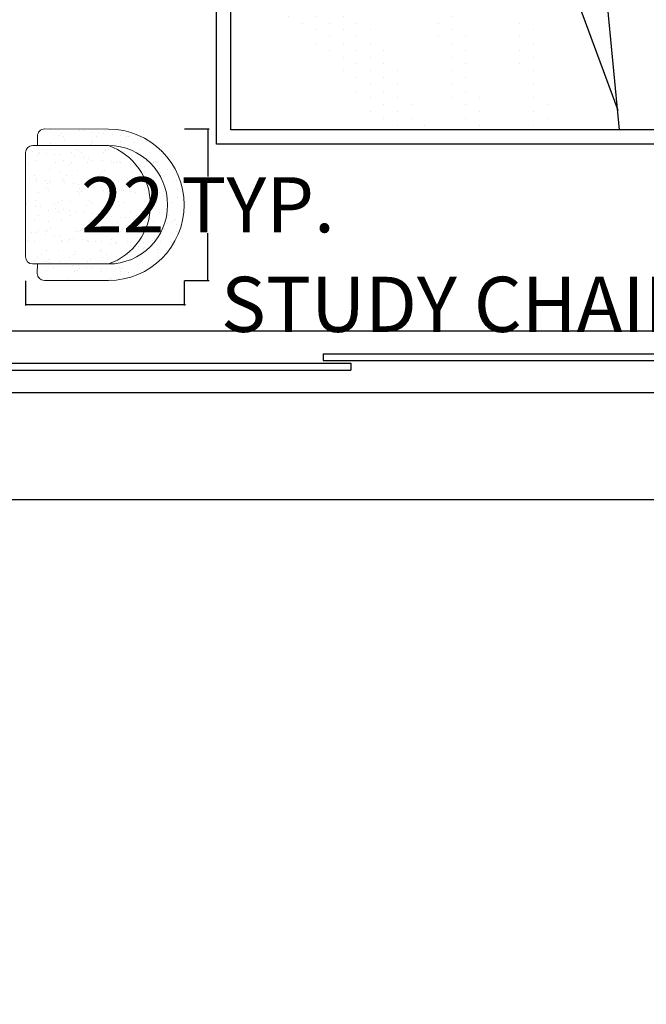
# Model space of a CAD drawing. Units: inches. Extents: x -48 to 50072, y 0 to 21068.
# Tile 60 of 75: x 793 to 883, y 660 to 803. Entities that reach past the tile are written whole.
import ezdxf

# ---------------------------------------------------------------- set-up
doc = ezdxf.new("R2010")
doc.units = ezdxf.units.IN
doc.header["$MEASUREMENT"] = 0
for name, color, linetype, lineweight in [('A-ANNO-DIMS', 2, 'Continuous', 18), ('A-DOOR', 4, 'Continuous', 18), ('FURNITURE', 44, 'Continuous', 18)]:
    doc.layers.add(name, color=color, linetype=linetype, lineweight=lineweight)
doc.layers.add('Layer3', color=176, linetype='Continuous')
doc.styles.get("Standard").update_dxf_attribs({"font": 'arial.ttf'})
doc.dimstyles.get("Standard").update_dxf_attribs({"dimtxt": 8, "dimasz": 0.18, "dimexe": 0.18, "dimexo": 0.0625, "dimgap": 0.09, "dimtad": 0, "dimtih": 1, "dimtoh": 1, "dimdec": 1, "dimzin": 0, "dimdsep": 46, "dimlunit": 4, "dimtxsty": 'Standard', "dimblk": 'ARCHTICK', "dimcen": 0.09, "dimadec": 0, "dimazin": 0, "dimtfac": 1, "dimtdec": 1, "dimtofl": 0, "dimtmove": 0, "dimatfit": 3, "dimldrblk": 'ARCHTICK', "dimfxl": 1, "dimtolj": 1, "dimtzin": 0, "dimarcsym": 0})

# ---------------------------------------------------------------- blocks, each defined once
blk = doc.blocks.new('fdsghhhhhhygr')
for p, q in [((41.77, 686.77), (41.77, 677.77)), ((144.77, 677.77), (144.77, 686.77))]:
    blk.add_line(p, q)
at = {"layer": 'Defpoints'}
for p, q in [((91.27, 683.47), (144.77, 683.47)), ((91.27, 683.47), (91.27, 682.47)), ((91.27, 682.47), (144.77, 682.47)), ((41.77, 682.07), (95.27, 682.07)), ((41.77, 681.07), (95.27, 681.07)), ((95.27, 682.07), (95.27, 681.07))]:
    blk.add_line(p, q, dxfattribs=at)
at = {"layer": 'Layer3'}
for p, q in [((41.77, 686.77), (144.77, 686.77)), ((144.77, 677.77), (41.77, 677.77))]:
    blk.add_line(p, q, dxfattribs=at)
blk = doc.blocks.new('nhrygfdu7yu')
at = {"layer": 'Defpoints'}
for p, q in [((1019.17, 828.61), (845.97, 828.61)), ((845.97, 801.61), (845.97, 828.61)), ((848.67, 804.31), (848.67, 828.61)), ((881.27, 716.83), (881.27, 828.61)), ((983.87, 828.61), (983.87, 716.83)), ((1016.47, 804.31), (1016.47, 828.61)), ((1019.17, 801.61), (1019.17, 828.61)), ((884.03, 719.53), (884.03, 827.53)), ((884.03, 827.53), (981.17, 827.53)), ((981.17, 827.53), (981.17, 719.53)), ((864.18, 805.04), (864.18, 824.84)), ((1000.24, 805.98), (1000.24, 825.78)), ((892.12, 822.13), (892.12, 801.97)), ((929.67, 822.13), (892.12, 822.13)), ((929.67, 822.13), (929.67, 801.78)), ((935.52, 822.13), (935.52, 801.78)), ((935.52, 822.13), (973.07, 822.13)), ((973.07, 822.13), (973.07, 801.97)), ((926.47, 818.07), (927.21, 812.5)), ((947.88, 818.06), (943.61, 812.45)), ((1010.72, 815.93), (989.15, 815.93)), ((874.65, 814.99), (853.09, 814.99)), ((927.21, 812.5), (925.82, 805.91)), ((934.43, 807.75), (933.36, 812.55)), ((943.61, 812.45), (939.55, 805.41)), ((914.58, 810.18), (913.28, 809.99)), ((919.69, 808.14), (914.58, 810.18)), ((923.4, 803.12), (919.69, 808.14)), ((935.49, 804.66), (934.43, 807.75)), ((881.07, 804.31), (848.67, 804.31)), ((881.07, 804.31), (881.07, 804.31)), ((916.07, 804.42), (910.77, 803.49)), ((919.78, 804.61), (916.07, 804.42)), ((923.4, 803.12), (919.78, 804.61)), ((925.82, 805.91), (923.4, 803.12)), ((938.59, 802.42), (935.49, 804.66)), ((939.55, 805.41), (938.59, 802.42)), ((938.59, 802.42), (945.53, 804.13)), ((945.53, 804.13), (951.08, 803.38)), ((984.07, 804.31), (1016.47, 804.31)), ((984.07, 804.31), (984.07, 804.31)), ((910.77, 803.49), (910.59, 803.15)), ((923.4, 803.12), (925.08, 798.67)), ((923.4, 803.12), (933.44, 802.1)), ((935.45, 803.17), (936.69, 800.13)), ((938.59, 802.42), (937.95, 797.34)), ((938.59, 802.42), (941.26, 799.01)), ((951.08, 803.38), (953.02, 802.3)), ((881.07, 801.61), (845.97, 801.61)), ((884.06, 801.97), (981.18, 801.97)), ((933.44, 802.1), (936.13, 800.15)), ((984.07, 801.61), (1019.17, 801.61)), ((925.08, 798.67), (923.96, 794.21)), ((936.13, 800.15), (936.78, 799.69)), ((936.69, 800.13), (937.65, 797.78)), ((941.26, 799.01), (944.78, 796.45)), ((937.86, 796.54), (937.22, 791.44)), ((944.78, 796.45), (949.8, 796.45)), ((981.13, 793.06), (883.98, 783.7)), ((923.96, 794.21), (921.07, 790.83)), ((906.36, 766.47), (977.44, 792.73)), ((976.41, 779.36), (976.41, 779.36)), ((978.98, 779.36), (978.98, 779.36)), ((962.27, 776.79), (962.27, 776.79)), ((964.84, 776.79), (964.84, 776.79)), ((967.41, 776.79), (967.41, 776.79)), ((969.98, 776.79), (969.98, 776.79)), ((972.55, 776.79), (972.55, 776.79)), ((975.13, 776.79), (975.13, 776.79)), ((977.7, 776.79), (977.7, 776.79)), ((980.27, 776.79), (980.27, 776.79)), ((950.69, 774.21), (950.69, 774.21)), ((953.27, 774.21), (953.27, 774.21)), ((955.84, 774.21), (955.84, 774.21)), ((958.41, 774.21), (958.41, 774.21)), ((960.98, 774.21), (960.98, 774.21)), ((963.55, 774.21), (963.55, 774.21)), ((966.13, 774.21), (966.13, 774.21)), ((968.7, 774.21), (968.7, 774.21)), ((941.69, 771.64), (941.69, 771.64)), ((944.27, 771.64), (944.27, 771.64)), ((946.84, 771.64), (946.84, 771.64)), ((949.41, 771.64), (949.41, 771.64)), ((951.98, 771.64), (951.98, 771.64)), ((954.55, 771.64), (954.55, 771.64)), ((935.26, 769.07), (935.26, 769.07)), ((937.84, 769.07), (937.84, 769.07)), ((940.41, 769.07), (940.41, 769.07)), ((942.98, 769.07), (942.98, 769.07)), ((928.83, 766.5), (928.83, 766.5)), ((931.41, 766.5), (931.41, 766.5)), ((933.98, 766.5), (933.98, 766.5)), ((936.55, 766.5), (936.55, 766.5)), ((975.13, 766.5), (975.13, 766.5)), ((977.7, 766.5), (977.7, 766.5)), ((980.27, 766.5), (980.27, 766.5)), ((924.98, 763.93), (924.98, 763.93)), ((927.55, 763.93), (927.55, 763.93)), ((930.12, 763.93), (930.12, 763.93)), ((963.55, 763.93), (963.55, 763.93)), ((966.13, 763.93), (966.13, 763.93)), ((968.7, 763.93), (968.7, 763.93)), ((971.27, 763.93), (971.27, 763.93)), ((973.84, 763.93), (973.84, 763.93)), ((976.41, 763.93), (976.41, 763.93)), ((978.98, 763.93), (978.98, 763.93)), ((921.12, 761.35), (921.12, 761.35)), ((923.69, 761.35), (923.69, 761.35)), ((954.55, 761.35), (954.55, 761.35)), ((957.12, 761.35), (957.12, 761.35)), ((959.7, 761.35), (959.7, 761.35)), ((962.27, 761.35), (962.27, 761.35)), ((964.84, 761.35), (964.84, 761.35)), ((967.41, 761.35), (967.41, 761.35)), ((969.98, 761.35), (969.98, 761.35)), ((972.55, 761.35), (972.55, 761.35)), ((975.13, 761.35), (975.13, 761.35)), ((917.26, 758.78), (917.26, 758.78)), ((919.83, 758.78), (919.83, 758.78)), ((945.55, 758.78), (945.55, 758.78)), ((948.12, 758.78), (948.12, 758.78)), ((950.69, 758.78), (950.69, 758.78)), ((953.27, 758.78), (953.27, 758.78)), ((955.84, 758.78), (955.84, 758.78)), ((958.41, 758.78), (958.41, 758.78)), ((960.98, 758.78), (960.98, 758.78)), ((963.55, 758.78), (963.55, 758.78)), ((913.4, 756.21), (913.4, 756.21)), ((915.98, 756.21), (915.98, 756.21)), ((941.69, 756.21), (941.69, 756.21)), ((944.27, 756.21), (944.27, 756.21)), ((946.84, 756.21), (946.84, 756.21)), ((949.41, 756.21), (949.41, 756.21)), ((951.98, 756.21), (951.98, 756.21)), ((954.55, 756.21), (954.55, 756.21)), ((957.12, 756.21), (957.12, 756.21)), ((980.27, 756.21), (980.27, 756.21)), ((909.55, 753.64), (909.55, 753.64)), ((912.12, 753.64), (912.12, 753.64)), ((935.26, 753.64), (935.26, 753.64)), ((937.84, 753.64), (937.84, 753.64)), ((940.41, 753.64), (940.41, 753.64)), ((942.98, 753.64), (942.98, 753.64)), ((945.55, 753.64), (945.55, 753.64)), ((948.12, 753.64), (948.12, 753.64)), ((976.41, 753.64), (976.41, 753.64)), ((978.98, 753.64), (978.98, 753.64)), ((905.69, 751.07), (905.69, 751.07)), ((908.26, 751.07), (908.26, 751.07)), ((931.41, 751.07), (931.41, 751.07)), ((933.98, 751.07), (933.98, 751.07)), ((936.55, 751.07), (936.55, 751.07)), ((939.12, 751.07), (939.12, 751.07)), ((941.69, 751.07), (941.69, 751.07)), ((944.27, 751.07), (944.27, 751.07)), ((969.98, 751.07), (969.98, 751.07)), ((972.55, 751.07), (972.55, 751.07)), ((975.13, 751.07), (975.13, 751.07)), ((977.7, 751.07), (977.7, 751.07)), ((980.27, 751.07), (980.27, 751.07)), ((904.4, 748.5), (904.4, 748.5)), ((927.55, 748.5), (927.55, 748.5)), ((930.12, 748.5), (930.12, 748.5)), ((932.69, 748.5), (932.69, 748.5)), ((935.26, 748.5), (935.26, 748.5)), ((937.84, 748.5), (937.84, 748.5)), ((940.41, 748.5), (940.41, 748.5)), ((966.13, 748.5), (966.13, 748.5)), ((968.7, 748.5), (968.7, 748.5)), ((971.27, 748.5), (971.27, 748.5)), ((973.84, 748.5), (973.84, 748.5)), ((976.41, 748.5), (976.41, 748.5)), ((978.98, 748.5), (978.98, 748.5)), ((900.55, 745.92), (900.55, 745.92)), ((903.12, 745.92), (903.12, 745.92)), ((923.69, 745.92), (923.69, 745.92)), ((926.26, 745.92), (926.26, 745.92)), ((928.83, 745.92), (928.83, 745.92)), ((931.41, 745.92), (931.41, 745.92)), ((933.98, 745.92), (933.98, 745.92)), ((962.27, 745.92), (962.27, 745.92)), ((964.84, 745.92), (964.84, 745.92)), ((967.41, 745.92), (967.41, 745.92)), ((969.98, 745.92), (969.98, 745.92)), ((972.55, 745.92), (972.55, 745.92)), ((975.13, 745.92), (975.13, 745.92)), ((977.7, 745.92), (977.7, 745.92)), ((896.69, 743.35), (896.69, 743.35)), ((899.26, 743.35), (899.26, 743.35)), ((919.83, 743.35), (919.83, 743.35)), ((922.41, 743.35), (922.41, 743.35)), ((924.98, 743.35), (924.98, 743.35)), ((927.55, 743.35), (927.55, 743.35)), ((930.12, 743.35), (930.12, 743.35)), ((932.69, 743.35), (932.69, 743.35)), ((960.98, 743.35), (960.98, 743.35)), ((963.55, 743.35), (963.55, 743.35)), ((966.13, 743.35), (966.13, 743.35)), ((968.7, 743.35), (968.7, 743.35)), ((971.27, 743.35), (971.27, 743.35)), ((973.84, 743.35), (973.84, 743.35)), ((895.4, 740.78), (895.4, 740.78)), ((915.98, 740.78), (915.98, 740.78)), ((918.55, 740.78), (918.55, 740.78)), ((921.12, 740.78), (921.12, 740.78)), ((923.69, 740.78), (923.69, 740.78)), ((926.26, 740.78), (926.26, 740.78)), ((928.83, 740.78), (928.83, 740.78)), ((957.12, 740.78), (957.12, 740.78)), ((959.7, 740.78), (959.7, 740.78)), ((962.27, 740.78), (962.27, 740.78)), ((964.84, 740.78), (964.84, 740.78)), ((967.41, 740.78), (967.41, 740.78)), ((969.98, 740.78), (969.98, 740.78)), ((891.54, 738.21), (891.54, 738.21)), ((894.12, 738.21), (894.12, 738.21)), ((914.69, 738.21), (914.69, 738.21)), ((917.26, 738.21), (917.26, 738.21)), ((919.83, 738.21), (919.83, 738.21)), ((922.41, 738.21), (922.41, 738.21)), ((924.98, 738.21), (924.98, 738.21)), ((955.84, 738.21), (955.84, 738.21)), ((958.41, 738.21), (958.41, 738.21)), ((960.98, 738.21), (960.98, 738.21)), ((963.55, 738.21), (963.55, 738.21)), ((966.13, 738.21), (966.13, 738.21)), ((887.69, 735.64), (887.69, 735.64)), ((890.26, 735.64), (890.26, 735.64)), ((910.83, 735.64), (910.83, 735.64)), ((913.4, 735.64), (913.4, 735.64)), ((915.98, 735.64), (915.98, 735.64)), ((918.55, 735.64), (918.55, 735.64)), ((921.12, 735.64), (921.12, 735.64)), ((951.98, 735.64), (951.98, 735.64)), ((954.55, 735.64), (954.55, 735.64)), ((957.12, 735.64), (957.12, 735.64)), ((959.7, 735.64), (959.7, 735.64)), ((962.27, 735.64), (962.27, 735.64)), ((964.84, 735.64), (964.84, 735.64)), ((886.4, 733.07), (886.4, 733.07)), ((888.97, 733.07), (888.97, 733.07)), ((909.55, 733.07), (909.55, 733.07)), ((912.12, 733.07), (912.12, 733.07)), ((914.69, 733.07), (914.69, 733.07)), ((917.26, 733.07), (917.26, 733.07)), ((919.83, 733.07), (919.83, 733.07)), ((950.69, 733.07), (950.69, 733.07)), ((953.27, 733.07), (953.27, 733.07)), ((955.84, 733.07), (955.84, 733.07)), ((958.41, 733.07), (958.41, 733.07)), ((960.98, 733.07), (960.98, 733.07)), ((885.12, 730.49), (885.12, 730.49)), ((905.69, 730.49), (905.69, 730.49)), ((908.26, 730.49), (908.26, 730.49)), ((910.83, 730.49), (910.83, 730.49)), ((913.4, 730.49), (913.4, 730.49)), ((915.98, 730.49), (915.98, 730.49)), ((946.84, 730.49), (946.84, 730.49)), ((949.41, 730.49), (949.41, 730.49)), ((951.98, 730.49), (951.98, 730.49)), ((954.55, 730.49), (954.55, 730.49)), ((957.12, 730.49), (957.12, 730.49)), ((959.7, 730.49), (959.7, 730.49)), ((904.4, 727.92), (904.4, 727.92)), ((906.97, 727.92), (906.97, 727.92)), ((909.55, 727.92), (909.55, 727.92)), ((912.12, 727.92), (912.12, 727.92)), ((945.55, 727.92), (945.55, 727.92)), ((948.12, 727.92), (948.12, 727.92)), ((950.69, 727.92), (950.69, 727.92)), ((953.27, 727.92), (953.27, 727.92)), ((955.84, 727.92), (955.84, 727.92)), ((958.41, 727.92), (958.41, 727.92)), ((900.55, 725.35), (900.55, 725.35)), ((903.12, 725.35), (903.12, 725.35)), ((905.69, 725.35), (905.69, 725.35)), ((908.26, 725.35), (908.26, 725.35)), ((910.83, 725.35), (910.83, 725.35)), ((944.27, 725.35), (944.27, 725.35)), ((946.84, 725.35), (946.84, 725.35)), ((949.41, 725.35), (949.41, 725.35)), ((951.98, 725.35), (951.98, 725.35)), ((954.55, 725.35), (954.55, 725.35)), ((899.26, 722.78), (899.26, 722.78)), ((901.83, 722.78), (901.83, 722.78)), ((904.4, 722.78), (904.4, 722.78)), ((906.97, 722.78), (906.97, 722.78)), ((942.98, 722.78), (942.98, 722.78)), ((945.55, 722.78), (945.55, 722.78)), ((948.12, 722.78), (948.12, 722.78)), ((950.69, 722.78), (950.69, 722.78)), ((953.27, 722.78), (953.27, 722.78)), ((981.17, 719.53), (884.03, 719.53)), ((895.4, 720.21), (895.4, 720.21)), ((897.97, 720.21), (897.97, 720.21)), ((900.55, 720.21), (900.55, 720.21)), ((903.12, 720.21), (903.12, 720.21)), ((905.69, 720.21), (905.69, 720.21)), ((939.12, 720.21), (939.12, 720.21)), ((941.69, 720.21), (941.69, 720.21)), ((944.27, 720.21), (944.27, 720.21)), ((946.84, 720.21), (946.84, 720.21)), ((949.41, 720.21), (949.41, 720.21)), ((951.98, 720.21), (951.98, 720.21)), ((983.87, 716.83), (881.27, 716.83))]:
    blk.add_line(p, q, dxfattribs=at)
for centre, radius in [((864.18, 814.99), 8.1), ((1000.24, 815.93), 8.1), ((864.18, 814.99), 6.48), ((1000.24, 815.93), 6.48)]:
    blk.add_circle(centre, radius, dxfattribs=at)
for centre, radius, start, end in [((924.05, 817.43), 1.94, 297.2902, 3.2455), ((926.67, 817.58), 0.687, 51.1864, 183.2455), ((924.75, 815.18), 3.76, 45.8726, 51.1864), ((929.07, 819.63), 2.44, 225.8726, 232.4713), ((940.16, 834.08), 20.66, 232.4713, 233.7837), ((906.88, 788.64), 35.67, 52.7849, 53.7837), ((943.53, 820.78), 4.28, 292.7069, 308.5854), ((948.22, 814.9), 3.25, 110.3452, 128.5854), ((947.75, 816.16), 1.9, 86.0516, 110.3452), ((948.43, 816.91), 0.765, 126.5792, 169.5926), ((947.87, 817.82), 0.239, 13.2808, 86.0516), ((947.77, 817.8), 0.34, 306.5792, 13.2808), ((848.26, 964.34), 167.25, 296.4147, 297.2902), ((921.35, 807.68), 11.75, 46.4776, 52.7849), ((926.56, 813.17), 4.18, 35.8936, 46.4776), ((928.96, 814.91), 1.22, 351.9508, 35.8936), ((848.62, 1074.38), 275.09, 289.0836, 290.1287), ((927.73, 858.54), 45.2, 290.1287, 292.7069), ((951.77, 816.3), 4.17, 169.5926, 177.2714), ((948.44, 816.46), 0.826, 177.2714, 194.5709), ((949.69, 816.78), 2.12, 194.5709, 206.8179), ((964.76, 824.4), 19.01, 206.8179, 210.9056), ((1072.97, 521.35), 329.5, 117.4999, 117.8482), ((971.1, 717.04), 108.88, 116.4147, 117.4999), ((932.62, 814.39), 2.47, 171.9508, 202.4162), ((980.52, 834.15), 54.29, 202.4162, 205.0529), ((883.03, 974.91), 169.83, 286.6085, 289.0836), ((957.44, 820.02), 10.47, 210.9056, 219.7005), ((901.77, 841.65), 33.68, 290.7486, 297.4921), ((771.78, 1091.44), 315.27, 297.4921, 297.8482), ((929.77, 818.2), 6.29, 280.7366, 286.6085), ((946.01, 810.53), 4.37, 26.0735, 39.7005), ((940.41, 807.79), 10.61, 17.8396, 26.0735), ((905.47, 831.87), 23.22, 282.6252, 290.7486), ((1013.86, 849.73), 91.09, 205.0529, 207.0884), ((847.55, 777.91), 108.16, 15.2625, 17.8396), ((908.02, 808.45), 0.313, 121.6917, 179.0386), ((908.61, 808.44), 0.905, 179.0386, 229.4914), ((909.3, 806.38), 2.75, 103.0402, 121.6917), ((909.41, 805.91), 3.23, 86.6119, 103.0402), ((909.8, 812.53), 3.4, 266.6119, 282.6252), ((1008.01, 846.74), 84.52, 207.0884, 209.936), ((905.38, 804.66), 4.08, 26.3332, 49.4914), ((780.21, 742.7), 143.74, 25.1732, 26.3332), ((866.04, 782.95), 89, 13.841, 15.2625), ((924.73, 798.79), 11.57, 22.2355, 29.936), ((981.05, 811.29), 29.45, 193.841, 196.3122), ((901.51, 799.71), 9.71, 20.7081, 25.1732), ((883.04, 792.73), 29.45, 18.2369, 20.7081), ((962.1, 805.74), 9.71, 196.3122, 200.7773), ((1087.42, 853.29), 143.74, 200.7773, 201.9373), ((995.54, 829.8), 89, 198.2369, 199.6584), ((1013.59, 836.25), 108.16, 199.6584, 202.2355), ((957.87, 801.11), 4.08, 201.9373, 225.0955), ((938.8, 798.25), 1.24, 202.2355, 252.8133), ((938.36, 796.82), 0.252, 289.3799, 72.8133), ((955.69, 773.98), 23.22, 98.2293, 106.3527), ((952.85, 793.6), 3.4, 82.216, 98.2293), ((953.75, 800.17), 3.23, 262.216, 278.6443), ((953.82, 799.69), 2.75, 278.6443, 297.2959), ((954.35, 797.58), 0.905, 354.6428, 45.0955), ((954.94, 797.53), 0.313, 297.2959, 354.6428), ((923.29, 799.33), 10.61, 202.2355, 210.4694), ((993.31, 637.11), 169.83, 111.0043, 113.4795), ((880.68, 777.46), 54.29, 18.0203, 19.3448), ((934.7, 789.77), 6.29, 98.1216, 111.0043), ((934.31, 792.46), 3.58, 85.4882, 98.1216), ((934.9, 799.87), 3.85, 265.4882, 277.6784), ((934.12, 805.65), 9.69, 277.6784, 284.8807), ((939.32, 786.09), 10.56, 97.9822, 104.8807), ((938.1, 794.73), 1.83, 85.7407, 97.9822), ((938.28, 797.05), 0.497, 265.7407, 289.3799), ((1069.09, 504.93), 315.27, 113.0962, 113.4523), ((958.63, 763.95), 33.68, 106.3527, 113.0962), ((917.92, 796.17), 4.37, 210.4694, 224.0964), ((907.26, 785.84), 10.47, 35.3015, 44.0964), ((929.96, 793.49), 2.47, 347.5549, 18.0203), ((933.57, 792.7), 1.22, 167.5549, 211.4977), ((899.06, 893.51), 108.88, 292.0188, 293.104), ((812.48, 1096.43), 329.5, 293.104, 293.4523), ((900.29, 780.91), 19.01, 31.2138, 35.3015), ((1035.25, 540.56), 275.09, 113.4795, 114.5246), ((936.09, 794.24), 4.18, 211.4977, 222.0817), ((941.71, 799.32), 11.75, 222.0817, 228.389), ((938.27, 789.81), 1.94, 112.8944, 178.8496), ((1002.58, 637.52), 167.25, 112.0188, 112.8944), ((916, 789.63), 0.765, 310.9751, 353.9885), ((914.73, 789.66), 2.12, 18.9668, 31.2138), ((915.96, 790.08), 0.826, 1.6673, 18.9668), ((912.62, 789.98), 4.17, 353.9885, 1.6673), ((916.05, 791.65), 3.25, 294.7411, 312.9813), ((921.18, 786.14), 4.28, 117.1028, 132.9813), ((939.83, 749.71), 45.2, 114.5246, 117.1028), ((957.59, 817.2), 35.67, 228.389, 229.3878), ((920.93, 774.44), 20.66, 48.0754, 49.3878), ((933.1, 787.99), 2.44, 41.4767, 48.0754), ((937.75, 792.1), 3.76, 221.4767, 226.7905), ((935.64, 789.86), 0.687, 226.7905, 358.8496), ((916.73, 788.79), 0.34, 130.9751, 197.6767), ((916.63, 788.76), 0.239, 197.6767, 270.4475), ((916.62, 790.42), 1.9, 270.4475, 294.7411)]:
    blk.add_arc(centre, radius, start, end, dxfattribs=at)
blk.add_ellipse((874.1, 762.91), major_axis=(32.71, 0), ratio=0.667085, start_param=0.16392, end_param=1.263761, dxfattribs=at)
blk = doc.blocks.new('CHAIR-STUDY')
for p, q in [((2.76, 21.97), (12.03, 21.96)), ((3.67, 21.9, 13.84), (3.67, 21.9, 13.84)), ((6.44, 21.95, 13.84), (6.44, 21.95, 13.84)), ((7.77, 21.75, 13.84), (7.77, 21.75, 13.84)), ((8.5, 21.68, 13.84), (8.5, 21.68, 13.84)), ((9.74, 21.52, 13.84), (9.74, 21.52, 13.84)), ((11.66, 21.77, 13.84), (11.66, 21.77, 13.84)), ((1.73, 20.94), (1.73, 19.57)), ((1.74, 20.38, 13.84), (1.74, 20.38, 13.84)), ((4.87, 21.05, 13.84), (4.87, 21.05, 13.84)), ((5.15, 21.3, 13.84), (5.15, 21.3, 13.84)), ((5.52, 20.9, 13.84), (5.52, 20.9, 13.84)), ((5.63, 20.39, 13.84), (5.63, 20.39, 13.84)), ((9.61, 20.34, 13.84), (9.61, 20.34, 13.84)), ((10.25, 20.89, 13.84), (10.25, 20.89, 13.84)), ((10.53, 21.41, 13.84), (10.53, 21.41, 13.84)), ((11.24, 21.36, 13.84), (11.24, 21.36, 13.84)), ((12.59, 21.14, 13.84), (12.59, 21.14, 13.84)), ((13.71, 20.2, 13.84), (13.71, 20.2, 13.84)), ((13.83, 20.98, 13.84), (13.83, 20.98, 13.84)), ((14.62, 20.87, 13.84), (14.62, 20.87, 13.84)), ((14.99, 20.88, 13.84), (14.99, 20.88, 13.84)), ((15.81, 20.02, 13.84), (15.81, 20.02, 13.84)), ((16.68, 20.6, 13.84), (16.68, 20.6, 13.84)), ((17.6, 20.21, 13.84), (17.6, 20.21, 13.84)), ((0.15, 18.84, 13.84), (0.15, 18.84, 13.84)), ((0.94, 18.74, 13.84), (0.94, 18.74, 13.84)), ((1.04, 19.57), (12.03, 19.56)), ((1.87, 18.57, 13.84), (1.87, 18.57, 13.84)), ((2.51, 18.98, 13.84), (2.51, 18.98, 13.84)), ((3.55, 19.84, 13.84), (3.55, 19.84, 13.84)), ((3.57, 18.97, 13.84), (3.57, 18.97, 13.84)), ((6.6, 18.56, 13.84), (6.6, 18.56, 13.84)), ((7.24, 18.97, 13.84), (7.24, 18.97, 13.84)), ((7.68, 18.82, 13.84), (7.68, 18.82, 13.84)), ((9.44, 19.71, 13.84), (9.44, 19.71, 13.84)), ((9.72, 19.97, 13.84), (9.72, 19.97, 13.84)), ((11.57, 18.84, 13.84), (11.57, 18.84, 13.84)), ((11.97, 18.96, 13.84), (11.97, 18.96, 13.84)), ((14.29, 18.64, 13.84), (14.29, 18.64, 13.84)), ((15.54, 18.79, 13.84), (15.54, 18.79, 13.84)), ((16.71, 18.96, 13.84), (16.71, 18.96, 13.84)), ((19.65, 18.64, 13.84), (19.65, 18.64, 13.84)), ((0.01, 18.54), (0, 3.44)), ((1.64, 17.45, 13.84), (1.64, 17.45, 13.84)), ((1.76, 18.19, 13.84), (1.76, 18.19, 13.84)), ((2.04, 18.45, 13.84), (2.04, 18.45, 13.84)), ((3.01, 18.47, 13.84), (3.01, 18.47, 13.84)), ((4.24, 18.3, 13.84), (4.24, 18.3, 13.84)), ((5.03, 18.2, 13.84), (5.03, 18.2, 13.84)), ((5.53, 17.47, 13.84), (5.53, 17.47, 13.84)), ((7.1, 17.93, 13.84), (7.1, 17.93, 13.84)), ((8.12, 18.5, 13.84), (8.12, 18.5, 13.84)), ((8.34, 17.77, 13.84), (8.34, 17.77, 13.84)), ((9.13, 17.66, 13.84), (9.13, 17.66, 13.84)), ((9.51, 17.42, 13.84), (9.51, 17.42, 13.84)), ((11.19, 17.39, 13.84), (11.19, 17.39, 13.84)), ((11.33, 18.56, 13.84), (11.33, 18.56, 13.84)), ((12.43, 17.23, 13.84), (12.43, 17.23, 13.84)), ((12.69, 17.17, 13.84), (12.69, 17.17, 13.84)), ((13.62, 17.27, 13.84), (13.62, 17.27, 13.84)), ((14.01, 18.38, 13.84), (14.01, 18.38, 13.84)), ((16.07, 18.55, 13.84), (16.07, 18.55, 13.84)), ((17.5, 17.29, 13.84), (17.5, 17.29, 13.84)), ((18.86, 17.3, 13.84), (18.86, 17.3, 13.84)), ((0.44, 16.98, 13.84), (0.44, 16.98, 13.84)), ((3.48, 16.04, 13.84), (3.48, 16.04, 13.84)), ((4.29, 17.09, 13.84), (4.29, 17.09, 13.84)), ((6.33, 16.86, 13.84), (6.33, 16.86, 13.84)), ((6.61, 17.12, 13.84), (6.61, 17.12, 13.84)), ((7.58, 15.89, 13.84), (7.58, 15.89, 13.84)), ((9.02, 17.09, 13.84), (9.02, 17.09, 13.84)), ((11.18, 15.78, 13.84), (11.18, 15.78, 13.84)), ((11.47, 15.91, 13.84), (11.47, 15.91, 13.84)), ((13.22, 17.12, 13.84), (13.22, 17.12, 13.84)), ((13.76, 17.08, 13.84), (13.76, 17.08, 13.84)), ((15.28, 16.85, 13.84), (15.28, 16.85, 13.84)), ((15.45, 15.86, 13.84), (15.45, 15.86, 13.84)), ((16.52, 16.69, 13.84), (16.52, 16.69, 13.84)), ((17.26, 15.83, 13.84), (17.26, 15.83, 13.84)), ((17.31, 16.58, 13.84), (17.31, 16.58, 13.84)), ((18.49, 17.07, 13.84), (18.49, 17.07, 13.84)), ((18.58, 17.05, 13.84), (18.58, 17.05, 13.84)), ((19.37, 16.31, 13.84), (19.37, 16.31, 13.84)), ((19.55, 15.71, 13.84), (19.55, 15.71, 13.84)), ((20.61, 16.15, 13.84), (20.61, 16.15, 13.84)), ((21.4, 16.05, 13.84), (21.4, 16.05, 13.84)), ((0.64, 14.77, 13.84), (0.64, 14.77, 13.84)), ((1.28, 15.17, 13.84), (1.28, 15.17, 13.84)), ((1.55, 14.52, 13.84), (1.55, 14.52, 13.84)), ((1.61, 14.72, 13.84), (1.61, 14.72, 13.84)), ((2.84, 14.55, 13.84), (2.84, 14.55, 13.84)), ((3.63, 14.45, 13.84), (3.63, 14.45, 13.84)), ((5.01, 15.65, 13.84), (5.01, 15.65, 13.84)), ((5.37, 14.76, 13.84), (5.37, 14.76, 13.84)), ((5.44, 14.54, 13.84), (5.44, 14.54, 13.84)), ((6.01, 15.17, 13.84), (6.01, 15.17, 13.84)), ((9.41, 14.49, 13.84), (9.41, 14.49, 13.84)), ((9.58, 14.31, 13.84), (9.58, 14.31, 13.84)), ((10.1, 14.75, 13.84), (10.1, 14.75, 13.84)), ((10.75, 15.16, 13.84), (10.75, 15.16, 13.84)), ((10.9, 15.52, 13.84), (10.9, 15.52, 13.84)), ((13.52, 14.34, 13.84), (13.52, 14.34, 13.84)), ((14.84, 14.74, 13.84), (14.84, 14.74, 13.84)), ((15.48, 15.15, 13.84), (15.48, 15.15, 13.84)), ((15.75, 14.45, 13.84), (15.75, 14.45, 13.84)), ((17.41, 14.36, 13.84), (17.41, 14.36, 13.84)), ((19.57, 14.73, 13.84), (19.57, 14.73, 13.84)), ((20.21, 15.14, 13.84), (20.21, 15.14, 13.84)), ((21.39, 14.31, 13.84), (21.39, 14.31, 13.84)), ((21.83, 14.5, 13.84), (21.83, 14.5, 13.84)), ((3.06, 13.29, 13.84), (3.06, 13.29, 13.84)), ((3.21, 14, 13.84), (3.21, 14, 13.84)), ((3.38, 13.11, 13.84), (3.38, 13.11, 13.84)), ((3.49, 14.26, 13.84), (3.49, 14.26, 13.84)), ((5.7, 14.18, 13.84), (5.7, 14.18, 13.84)), ((6.93, 14.01, 13.84), (6.93, 14.01, 13.84)), ((7.49, 12.96, 13.84), (7.49, 12.96, 13.84)), ((7.72, 13.91, 13.84), (7.72, 13.91, 13.84)), ((7.8, 13.28, 13.84), (7.8, 13.28, 13.84)), ((8.06, 12.93, 13.84), (8.06, 12.93, 13.84)), ((9.79, 13.64, 13.84), (9.79, 13.64, 13.84)), ((11.03, 13.48, 13.84), (11.03, 13.48, 13.84)), ((11.37, 12.98, 13.84), (11.37, 12.98, 13.84)), ((11.82, 13.37, 13.84), (11.82, 13.37, 13.84)), ((12.53, 13.27, 13.84), (12.53, 13.27, 13.84)), ((13.88, 13.1, 13.84), (13.88, 13.1, 13.84)), ((14.14, 12.98, 13.84), (14.14, 12.98, 13.84)), ((15.12, 12.94, 13.84), (15.12, 12.94, 13.84)), ((15.35, 12.93, 13.84), (15.35, 12.93, 13.84)), ((15.47, 14.19, 13.84), (15.47, 14.19, 13.84)), ((17.26, 13.26, 13.84), (17.26, 13.26, 13.84)), ((20.04, 12.86, 13.84), (20.04, 12.86, 13.84)), ((20.32, 13.11, 13.84), (20.32, 13.11, 13.84)), ((22, 13.25, 13.84), (22, 13.25, 13.84)), ((1.45, 11.59, 13.84), (1.45, 11.59, 13.84)), ((1.89, 12.79, 13.84), (1.89, 12.79, 13.84)), ((5.34, 11.61, 13.84), (5.34, 11.61, 13.84)), ((6.46, 11.46, 13.84), (6.46, 11.46, 13.84)), ((7.78, 12.67, 13.84), (7.78, 12.67, 13.84)), ((9.32, 11.56, 13.84), (9.32, 11.56, 13.84)), ((12.63, 11.59, 13.84), (12.63, 11.59, 13.84)), ((15.91, 12.83, 13.84), (15.91, 12.83, 13.84)), ((17.31, 11.43, 13.84), (17.31, 11.43, 13.84)), ((17.97, 12.56, 13.84), (17.97, 12.56, 13.84)), ((18.71, 11.64, 13.84), (18.71, 11.64, 13.84)), ((19.21, 12.4, 13.84), (19.21, 12.4, 13.84)), ((19.46, 12.78, 13.84), (19.46, 12.78, 13.84)), ((20, 12.29, 13.84), (20, 12.29, 13.84)), ((22.06, 12.02, 13.84), (22.06, 12.02, 13.84)), ((0.05, 11.37, 13.84), (0.05, 11.37, 13.84)), ((0.1, 11.15, 13.84), (0.1, 11.15, 13.84)), ((0.21, 10.96, 13.84), (0.21, 10.96, 13.84)), ((0.38, 11.41, 13.84), (0.38, 11.41, 13.84)), ((1.44, 10.8, 13.84), (1.44, 10.8, 13.84)), ((2.23, 10.7, 13.84), (2.23, 10.7, 13.84)), ((3.28, 10.18, 13.84), (3.28, 10.18, 13.84)), ((4.14, 10.95, 13.84), (4.14, 10.95, 13.84)), ((4.3, 10.43, 13.84), (4.3, 10.43, 13.84)), ((4.78, 11.36, 13.84), (4.78, 11.36, 13.84)), ((4.95, 10.07, 13.84), (4.95, 10.07, 13.84)), ((5.53, 10.26, 13.84), (5.53, 10.26, 13.84)), ((6.32, 10.16, 13.84), (6.32, 10.16, 13.84)), ((7.39, 10.04, 13.84), (7.39, 10.04, 13.84)), ((8.88, 10.94, 13.84), (8.88, 10.94, 13.84)), ((9.52, 11.35, 13.84), (9.52, 11.35, 13.84)), ((11.03, 10.12, 13.84), (11.03, 10.12, 13.84)), ((11.28, 10.05, 13.84), (11.28, 10.05, 13.84)), ((12.35, 11.34, 13.84), (12.35, 11.34, 13.84)), ((13.42, 11.41, 13.84), (13.42, 11.41, 13.84)), ((13.61, 10.93, 13.84), (13.61, 10.93, 13.84)), ((14.25, 11.34, 13.84), (14.25, 11.34, 13.84)), ((15.26, 10, 13.84), (15.26, 10, 13.84)), ((16.92, 10, 13.84), (16.92, 10, 13.84)), ((17.2, 10.26, 13.84), (17.2, 10.26, 13.84)), ((18.34, 10.93, 13.84), (18.34, 10.93, 13.84)), ((18.99, 11.33, 13.84), (18.99, 11.33, 13.84)), ((21.29, 11.38, 13.84), (21.29, 11.38, 13.84)), ((1.36, 8.66, 13.84), (1.36, 8.66, 13.84)), ((1.84, 9.48, 13.84), (1.84, 9.48, 13.84)), ((3.34, 8.6, 13.84), (3.34, 8.6, 13.84)), ((4.67, 9.81, 13.84), (4.67, 9.81, 13.84)), ((5.24, 8.68, 13.84), (5.24, 8.68, 13.84)), ((6.57, 9.47, 13.84), (6.57, 9.47, 13.84)), ((8.39, 9.89, 13.84), (8.39, 9.89, 13.84)), ((9.22, 8.63, 13.84), (9.22, 8.63, 13.84)), ((9.52, 8.74, 13.84), (9.52, 8.74, 13.84)), ((9.62, 9.72, 13.84), (9.62, 9.72, 13.84)), ((10.41, 9.62, 13.84), (10.41, 9.62, 13.84)), ((11.3, 9.46, 13.84), (11.3, 9.46, 13.84)), ((12.48, 9.35, 13.84), (12.48, 9.35, 13.84)), ((13.72, 9.19, 13.84), (13.72, 9.19, 13.84)), ((14.51, 9.08, 13.84), (14.51, 9.08, 13.84)), ((15.6, 8.79, 13.84), (15.6, 8.79, 13.84)), ((16.04, 9.46, 13.84), (16.04, 9.46, 13.84)), ((16.57, 8.81, 13.84), (16.57, 8.81, 13.84)), ((17.81, 8.65, 13.84), (17.81, 8.65, 13.84)), ((19.36, 9.86, 13.84), (19.36, 9.86, 13.84)), ((20.77, 9.45, 13.84), (20.77, 9.45, 13.84)), ((21.49, 8.67, 13.84), (21.49, 8.67, 13.84)), ((21.77, 8.92, 13.84), (21.77, 8.92, 13.84)), ((1.83, 7.22, 13.84), (1.83, 7.22, 13.84)), ((2.92, 7.15, 13.84), (2.92, 7.15, 13.84)), ((3.19, 7.25, 13.84), (3.19, 7.25, 13.84)), ((3.56, 7.55, 13.84), (3.56, 7.55, 13.84)), ((7.91, 7.27, 13.84), (7.91, 7.27, 13.84)), ((8.29, 7.55, 13.84), (8.29, 7.55, 13.84)), ((9.24, 8.48, 13.84), (9.24, 8.48, 13.84)), ((13.02, 7.54, 13.84), (13.02, 7.54, 13.84)), ((13.33, 8.48, 13.84), (13.33, 8.48, 13.84)), ((13.81, 7.15, 13.84), (13.81, 7.15, 13.84)), ((14.09, 7.4, 13.84), (14.09, 7.4, 13.84)), ((17.22, 8.5, 13.84), (17.22, 8.5, 13.84)), ((17.76, 7.53, 13.84), (17.76, 7.53, 13.84)), ((18.6, 8.54, 13.84), (18.6, 8.54, 13.84)), ((20.17, 7.46, 13.84), (20.17, 7.46, 13.84)), ((20.66, 8.27, 13.84), (20.66, 8.27, 13.84)), ((21.2, 8.45, 13.84), (21.2, 8.45, 13.84)), ((21.9, 8.11, 13.84), (21.9, 8.11, 13.84)), ((0.04, 7.05, 13.84), (0.04, 7.05, 13.84)), ((0.23, 5.75, 13.84), (0.23, 5.75, 13.84)), ((0.83, 6.95, 13.84), (0.83, 6.95, 13.84)), ((1.26, 5.73, 13.84), (1.26, 5.73, 13.84)), ((1.55, 6.96, 13.84), (1.55, 6.96, 13.84)), ((2.9, 6.68, 13.84), (2.9, 6.68, 13.84)), ((4.13, 6.51, 13.84), (4.13, 6.51, 13.84)), ((4.92, 6.41, 13.84), (4.92, 6.41, 13.84)), ((5.15, 5.75, 13.84), (5.15, 5.75, 13.84)), ((6.4, 5.88, 13.84), (6.4, 5.88, 13.84)), ((6.99, 6.14, 13.84), (6.99, 6.14, 13.84)), ((7.29, 7.11, 13.84), (7.29, 7.11, 13.84)), ((7.65, 7.14, 13.84), (7.65, 7.14, 13.84)), ((8.22, 5.97, 13.84), (8.22, 5.97, 13.84)), ((9.01, 5.87, 13.84), (9.01, 5.87, 13.84)), ((11.18, 7.13, 13.84), (11.18, 7.13, 13.84)), ((12.38, 7.13, 13.84), (12.38, 7.13, 13.84)), ((12.48, 5.93, 13.84), (12.48, 5.93, 13.84)), ((15.16, 7.07, 13.84), (15.16, 7.07, 13.84)), ((17.12, 7.12, 13.84), (17.12, 7.12, 13.84)), ((18.37, 5.81, 13.84), (18.37, 5.81, 13.84)), ((18.65, 6.07, 13.84), (18.65, 6.07, 13.84)), ((19.27, 6.93, 13.84), (19.27, 6.93, 13.84)), ((21.85, 7.11, 13.84), (21.85, 7.11, 13.84)), ((0.61, 5.68, 13.84), (0.61, 5.68, 13.84)), ((3.09, 4.33, 13.84), (3.09, 4.33, 13.84)), ((4.8, 4.41, 13.84), (4.8, 4.41, 13.84)), ((5.34, 5.67, 13.84), (5.34, 5.67, 13.84)), ((6.12, 5.63, 13.84), (6.12, 5.63, 13.84)), ((9.13, 5.7, 13.84), (9.13, 5.7, 13.84)), ((10.08, 5.66, 13.84), (10.08, 5.66, 13.84)), ((10.69, 4.29, 13.84), (10.69, 4.29, 13.84)), ((10.97, 4.55, 13.84), (10.97, 4.55, 13.84)), ((11.08, 5.6, 13.84), (11.08, 5.6, 13.84)), ((12.31, 5.44, 13.84), (12.31, 5.44, 13.84)), ((13.1, 5.33, 13.84), (13.1, 5.33, 13.84)), ((13.23, 5.55, 13.84), (13.23, 5.55, 13.84)), ((14.81, 5.65, 13.84), (14.81, 5.65, 13.84)), ((15.17, 5.06, 13.84), (15.17, 5.06, 13.84)), ((16.41, 4.9, 13.84), (16.41, 4.9, 13.84)), ((17.05, 4.6, 13.84), (17.05, 4.6, 13.84)), ((17.12, 5.57, 13.84), (17.12, 5.57, 13.84)), ((17.2, 4.79, 13.84), (17.2, 4.79, 13.84)), ((19.26, 4.52, 13.84), (19.26, 4.52, 13.84)), ((19.54, 5.64, 13.84), (19.54, 5.64, 13.84)), ((20.5, 4.36, 13.84), (20.5, 4.36, 13.84)), ((21.1, 5.52, 13.84), (21.1, 5.52, 13.84)), ((1.49, 2.92, 13.84), (1.49, 2.92, 13.84)), ((1.69, 3.34, 13.84), (1.69, 3.34, 13.84)), ((2.33, 3.75, 13.84), (2.33, 3.75, 13.84)), ((3.29, 3.03, 13.84), (3.29, 3.03, 13.84)), ((6.42, 3.33, 13.84), (6.42, 3.33, 13.84)), ((7.06, 3.74, 13.84), (7.06, 3.74, 13.84)), ((7.2, 4.18, 13.84), (7.2, 4.18, 13.84)), ((9.37, 3.08, 13.84), (9.37, 3.08, 13.84)), ((11.09, 4.2, 13.84), (11.09, 4.2, 13.84)), ((11.16, 3.32, 13.84), (11.16, 3.32, 13.84)), ((11.8, 3.73, 13.84), (11.8, 3.73, 13.84)), ((15.07, 4.15, 13.84), (15.07, 4.15, 13.84)), ((15.26, 2.96, 13.84), (15.26, 2.96, 13.84)), ((15.54, 3.21, 13.84), (15.54, 3.21, 13.84)), ((15.89, 3.31, 13.84), (15.89, 3.31, 13.84)), ((16.53, 3.72, 13.84), (16.53, 3.72, 13.84)), ((19.17, 4, 13.84), (19.17, 4, 13.84)), ((1.03, 2.41), (12.01, 2.4)), ((1.16, 2.8, 13.84), (1.16, 2.8, 13.84)), ((1.72, 2.41), (1.71, 1.04)), ((2.73, 2.76, 13.84), (2.73, 2.76, 13.84)), ((3.01, 2.77, 13.84), (3.01, 2.77, 13.84)), ((3.52, 2.66, 13.84), (3.52, 2.66, 13.84)), ((4.11, 1.86, 13.84), (4.11, 1.86, 13.84)), ((5.05, 2.82, 13.84), (5.05, 2.82, 13.84)), ((5.59, 2.39, 13.84), (5.59, 2.39, 13.84)), ((6.82, 2.22, 13.84), (6.82, 2.22, 13.84)), ((7.57, 1.44, 13.84), (7.57, 1.44, 13.84)), ((7.61, 2.12, 13.84), (7.61, 2.12, 13.84)), ((7.85, 1.69, 13.84), (7.85, 1.69, 13.84)), ((8.85, 1.85, 13.84), (8.85, 1.85, 13.84)), ((9.03, 2.77, 13.84), (9.03, 2.77, 13.84)), ((9.68, 1.85, 13.84), (9.68, 1.85, 13.84)), ((10.91, 1.68, 13.84), (10.91, 1.68, 13.84)), ((11.7, 1.58, 13.84), (11.7, 1.58, 13.84)), ((13.14, 2.62, 13.84), (13.14, 2.62, 13.84)), ((13.58, 1.84, 13.84), (13.58, 1.84, 13.84)), ((13.94, 1.75, 13.84), (13.94, 1.75, 13.84)), ((17.02, 2.64, 13.84), (17.02, 2.64, 13.84)), ((2.74, 0.01), (12.01, 0)), ((3, 1.4, 13.84), (3, 1.4, 13.84)), ((6.25, 0.23, 13.84), (6.25, 0.23, 13.84)), ((7.1, 1.25, 13.84), (7.1, 1.25, 13.84)), ((10.99, 1.27, 13.84), (10.99, 1.27, 13.84)), ((12.14, 0.1, 13.84), (12.14, 0.1, 13.84)), ((12.42, 0.36, 13.84), (12.42, 0.36, 13.84)), ((13.77, 1.31, 13.84), (13.77, 1.31, 13.84)), ((14.97, 1.22, 13.84), (14.97, 1.22, 13.84)), ((15, 1.15, 13.84), (15, 1.15, 13.84)), ((15.8, 1.04, 13.84), (15.8, 1.04, 13.84))]:
    blk.add_line(p, q)
for centre, radius, start, end in [((2.76, 20.94), 1.03, 89.9486, 179.9486), ((12.02, 10.98), 10.98, 359.9486, 89.9486), ((1.04, 18.54), 1.03, 89.9486, 179.9486), ((9.02, 10.98), 9.09, 289.2386, 70.6585), ((12.02, 10.98), 8.58, 359.9486, 89.9486), ((12.02, 10.98), 10.98, 269.9486, 359.9486), ((12.02, 10.98), 8.58, 269.9486, 359.9486), ((1.03, 3.44), 1.03, 179.9486, 269.9486), ((2.74, 1.04), 1.03, 179.9486, 269.9486)]:
    blk.add_arc(centre, radius, start, end)
blk = doc.blocks.new('_ArchTick')
at = {"color": 0, "linetype": 'ByBlock', "const_width": 0.15}
blk.add_lwpolyline([(-0.5, -0.5), (0.5, 0.5)], dxfattribs=at)
blk = doc.blocks.new('*D60')
at = {"layer": 'A-ANNO-DIMS', "color": 0, "lineweight": -2, "transparency": 16777216}
for p, q in [((787.01, 748.4), (787.01, 732.83)), ((890.01, 748.4), (890.01, 732.83)), ((787.01, 733.01), (890.01, 733.01)), ((890.01, 733.01), (890.19, 733.01))]:
    blk.add_line(p, q, dxfattribs=at)
at = {"layer": 'Defpoints', "color": 0, "transparency": 16777216}
for p in [(787.01, 748.46), (890.01, 748.46), (890.01, 733.01)]:
    blk.add_point(p, dxfattribs=at)
at = {"layer": 'A-ANNO-DIMS', "color": 0, "lineweight": -2, "transparency": 16777216, "xscale": 0.18, "yscale": 0.18, "zscale": 0.18, "rotation": 180}
blk.add_blockref('_ArchTick', (787.01, 733.01), dxfattribs=at)
at = {"layer": 'A-ANNO-DIMS', "color": 0, "lineweight": -2, "transparency": 16777216, "xscale": 0.18, "yscale": 0.18, "zscale": 0.18}
blk.add_blockref('_ArchTick', (890.01, 733.01), dxfattribs=at)
at = {"layer": 'A-ANNO-DIMS', "color": 0, "transparency": 16777216, "insert": (960.35, 733.01), "char_height": 8, "attachment_point": 5}
blk.add_mtext('\\A1;SLIDING DOOR A 103 TYP.', dxfattribs=at)
blk = doc.blocks.new('*D80')
at = {"layer": 'A-ANNO-DIMS', "color": 0, "lineweight": -2, "transparency": 16777216}
for p, q in [((793.35, 764.7), (793.35, 761.13)), ((816.36, 764.7), (816.36, 761.13)), ((793.35, 761.31), (816.36, 761.31)), ((816.36, 761.31), (816.54, 761.31))]:
    blk.add_line(p, q, dxfattribs=at)
at = {"layer": 'Defpoints', "color": 0, "transparency": 16777216}
for p in [(793.35, 764.76), (816.36, 764.76), (816.36, 761.31)]:
    blk.add_point(p, dxfattribs=at)
at = {"layer": 'A-ANNO-DIMS', "color": 0, "lineweight": -2, "transparency": 16777216, "xscale": 0.18, "yscale": 0.18, "zscale": 0.18, "rotation": 180}
blk.add_blockref('_ArchTick', (793.35, 761.31), dxfattribs=at)
at = {"layer": 'A-ANNO-DIMS', "color": 0, "lineweight": -2, "transparency": 16777216, "xscale": 0.18, "yscale": 0.18, "zscale": 0.18}
blk.add_blockref('_ArchTick', (816.36, 761.31), dxfattribs=at)
at = {"layer": 'A-ANNO-DIMS', "color": 0, "transparency": 16777216, "insert": (875.51, 761.31), "char_height": 8, "attachment_point": 5}
blk.add_mtext('\\A1;STUDY CHAIR 23 TYP.', dxfattribs=at)
blk = doc.blocks.new('*D81')
at = {"layer": 'A-ANNO-DIMS', "color": 0, "lineweight": -2, "transparency": 16777216}
for p, q in [((816.42, 786.74), (819.99, 786.74)), ((819.81, 786.74), (819.81, 779.86)), ((819.81, 764.76), (819.81, 771.64)), ((816.42, 764.76), (819.99, 764.76))]:
    blk.add_line(p, q, dxfattribs=at)
at = {"layer": 'Defpoints', "color": 0, "transparency": 16777216}
for p in [(816.36, 786.74), (819.81, 786.74), (816.36, 764.76)]:
    blk.add_point(p, dxfattribs=at)
at = {"layer": 'A-ANNO-DIMS', "color": 0, "lineweight": -2, "transparency": 16777216, "xscale": 0.18, "yscale": 0.18, "zscale": 0.18}
for p, rotation in [((819.81, 786.74), 90), ((819.81, 764.76), 270)]:
    blk.add_blockref('_ArchTick', p, dxfattribs=dict(at, rotation=rotation))
at = {"layer": 'A-ANNO-DIMS', "color": 0, "transparency": 16777216, "insert": (819.81, 775.75), "char_height": 8, "attachment_point": 5}
blk.add_mtext('\\A1;22 TYP.', dxfattribs=at)
blk = doc.blocks.new('*D135')
at = {"layer": 'A-ANNO-DIMS', "color": 0, "lineweight": -2, "transparency": 16777216}
for p, q in [((763.26, 748.4), (763.26, 236.63)), ((909.26, 748.4), (909.26, 236.63)), ((763.26, 236.81), (827.71, 236.81)), ((909.26, 236.81), (844.81, 236.81))]:
    blk.add_line(p, q, dxfattribs=at)
at = {"layer": 'Defpoints', "color": 0, "transparency": 16777216}
for p in [(763.26, 748.46), (909.26, 748.46), (909.26, 236.81)]:
    blk.add_point(p, dxfattribs=at)
at = {"layer": 'A-ANNO-DIMS', "color": 0, "lineweight": -2, "transparency": 16777216, "xscale": 0.18, "yscale": 0.18, "zscale": 0.18, "rotation": 180}
blk.add_blockref('_ArchTick', (763.26, 236.81), dxfattribs=at)
at = {"layer": 'A-ANNO-DIMS', "color": 0, "lineweight": -2, "transparency": 16777216, "xscale": 0.18, "yscale": 0.18, "zscale": 0.18}
blk.add_blockref('_ArchTick', (909.26, 236.81), dxfattribs=at)
at = {"layer": 'A-ANNO-DIMS', "color": 0, "transparency": 16777216, "insert": (836.26, 236.81), "char_height": 8, "attachment_point": 5}
blk.add_mtext('\\A1;146', dxfattribs=at)
blk = doc.blocks.new('*D145')
at = {"layer": 'A-ANNO-DIMS', "color": 0, "lineweight": -2, "transparency": 16777216}
for p, q in [((961.2, 748.46), (710.63, 748.46)), ((710.81, 748.46), (710.81, 658.14)), ((710.81, 559.46), (710.81, 649.79)), ((961.2, 559.46), (710.63, 559.46))]:
    blk.add_line(p, q, dxfattribs=at)
at = {"layer": 'Defpoints', "color": 0, "transparency": 16777216}
for p in [(710.81, 748.46), (961.26, 748.46), (961.26, 559.46)]:
    blk.add_point(p, dxfattribs=at)
at = {"layer": 'A-ANNO-DIMS', "color": 0, "lineweight": -2, "transparency": 16777216, "xscale": 0.18, "yscale": 0.18, "zscale": 0.18}
for p, rotation in [((710.81, 748.46), 90), ((710.81, 559.46), 270)]:
    blk.add_blockref('_ArchTick', p, dxfattribs=dict(at, rotation=rotation))
at = {"layer": 'A-ANNO-DIMS', "color": 0, "transparency": 16777216, "insert": (710.81, 653.96), "char_height": 8, "attachment_point": 5}
blk.add_mtext('\\A1;189', dxfattribs=at)

msp = doc.modelspace()

# ---------------------------------------------------------------- block references
at = {"layer": 'A-DOOR'}
msp.add_blockref('fdsghhhhhhygr', (745.244, 70.689), dxfattribs=at)
at = {"layer": 'FURNITURE', "xscale": 0.7669307891904348, "yscale": 0.7669307891904348, "zscale": 0.7669307891904348, "rotation": 270}
msp.add_blockref('nhrygfdu7yu', (271.278, 1539.095), dxfattribs=at)
at = {"layer": 'FURNITURE'}
msp.add_blockref('CHAIR-STUDY', (793.355, 764.765), dxfattribs=at)

# ---------------------------------------------------------------- dimensions: what is measured, and where the dimension line sits
at = {"layer": 'A-ANNO-DIMS'}
for base, p1, p2, text, picture, middle in [((816.358, 761.309), (793.355, 764.76), (816.358, 764.76), 'STUDY CHAIR <> TYP.', '*D80', (875.509, 761.309)), ((890.012, 733.014), (787.01, 748.464), (890.012, 748.464), 'SLIDING DOOR A <> TYP.', '*D60', (960.347, 733.014))]:
    dim = msp.add_linear_dim(base=base, p1=p1, p2=p2, text=text, dimstyle='Standard', override={"dimdec": 0, "dimlfac": 1, "dimrnd": 0, "dimzin": 0, "dimdsep": 46, "dimlunit": 2}, dxfattribs=at)
    dim.commit()
    dim.dimension.update_dxf_attribs({"geometry": picture, "text_midpoint": middle})
dim = msp.add_linear_dim(base=(819.808, 786.738), p1=(816.358, 764.76), p2=(816.358, 786.738), angle=90, text='<> TYP.', dimstyle='Standard', override={"dimdec": 0, "dimlfac": 1, "dimrnd": 0, "dimzin": 0, "dimdsep": 46, "dimlunit": 2}, dxfattribs=at)
dim.commit()
dim.dimension.update_dxf_attribs({"geometry": '*D81', "text_midpoint": (819.808, 775.749)})
dim = msp.add_linear_dim(base=(710.811, 748.464), p1=(961.261, 559.464), p2=(961.261, 748.464), angle=90, dimstyle='Standard', override={"dimdec": 0, "dimlfac": 1, "dimrnd": 0, "dimzin": 0, "dimdsep": 46, "dimlunit": 2}, dxfattribs=at)
dim.commit()
dim.dimension.update_dxf_attribs({"geometry": '*D145', "text_midpoint": (710.811, 653.964)})
dim = msp.add_linear_dim(base=(909.261, 236.814), p1=(763.261, 748.464), p2=(909.261, 748.464), dimstyle='Standard', override={"dimdec": 0, "dimlfac": 1, "dimrnd": 0, "dimzin": 0, "dimdsep": 46, "dimlunit": 2}, dxfattribs=at)
dim.commit()
dim.dimension.update_dxf_attribs({"geometry": '*D135', "text_midpoint": (836.261, 236.814)})

doc.saveas('drawing.dxf')
